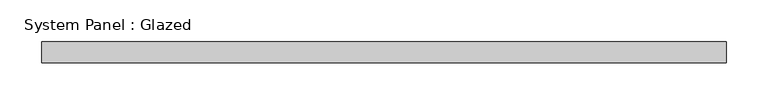
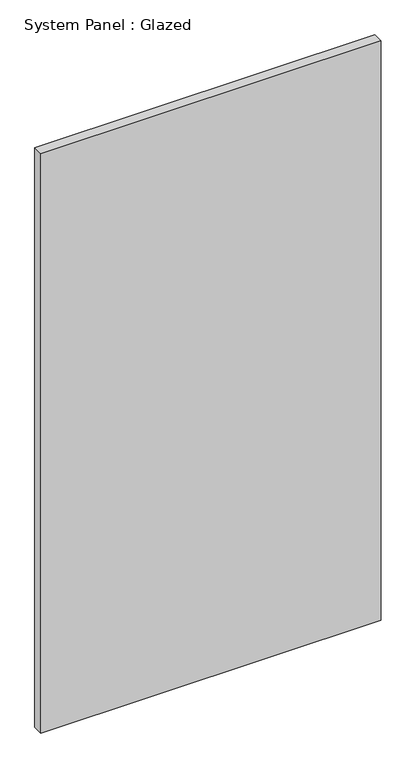
"""IFC4 building model written with IfcOpenShell, lengths in millimetres: plate geometry, System Panel : Glazed."""

from ifc_helpers import new_model, si_unit, origin, origin_with_axes, place, context, project, spatial, polyline, outline, extrude, source, transform, mapped, element, save


def system_panel_glazed_b88d7f0a(model_context):
    return source(origin(), model_context, "Body", "SweptSolid", [
        extrude(outline(polyline([(410.8680985, 19.05), (-410.8680985, 19.05), (-410.8680985, 44.45), (410.8680985, 44.45), (410.8680985, 19.05)])), origin_with_axes(), (0.0, 0.0, 1.0), 1478.5835026),
    ])


if __name__ == "__main__":
    model = new_model("IFC4")
    model_context = context("Model", 3, world=origin())
    ifc_project = project(units=[si_unit("LENGTHUNIT", "METRE", prefix="MILLI")], contexts=[model_context])
    site = spatial("IfcSite", under=ifc_project)
    building = spatial("IfcBuilding", under=site)
    placement = place(None, origin())
    system_panel_glazed_shape = system_panel_glazed_b88d7f0a(model_context)
    element("IfcPlate", 1, ObjectType="System Panel : Glazed", at=placement, inside=building, context=model_context, shape_type="MappedRepresentation", body=[
        mapped(system_panel_glazed_shape, transform((0.0, 0.0, 0.0), x_axis=(1.0, 0.0, 0.0), y_axis=(0.0, 1.0, 0.0), z_axis=(0.0, 0.0, 1.0))),
    ])
    save(model, "model.ifc")

# Revit data of these elements
# Type "System Panel : Glazed"
#   Construction Type Id = "GSP4R"
#   Analytic Construction = "1/8 in Pilkington single glazing"
#   Visual Light Transmittance = 0.9
#   Solar Heat Gain Coefficient = 0.86
#   Heat Transfer Coefficient (U) = 1.18115 BTU/(h·ft²·°F)
#   Define Thermal Properties by = 1
# Element 1 (IfcPlate, "System Panel : Glazed")
#   Materials on its faces: "Glass"
# Materials
#   "Glass": class "Glass", colour RGB 0 128 192, transparency 0.75, Description = "Soda Lime Glass", Cost = 0
